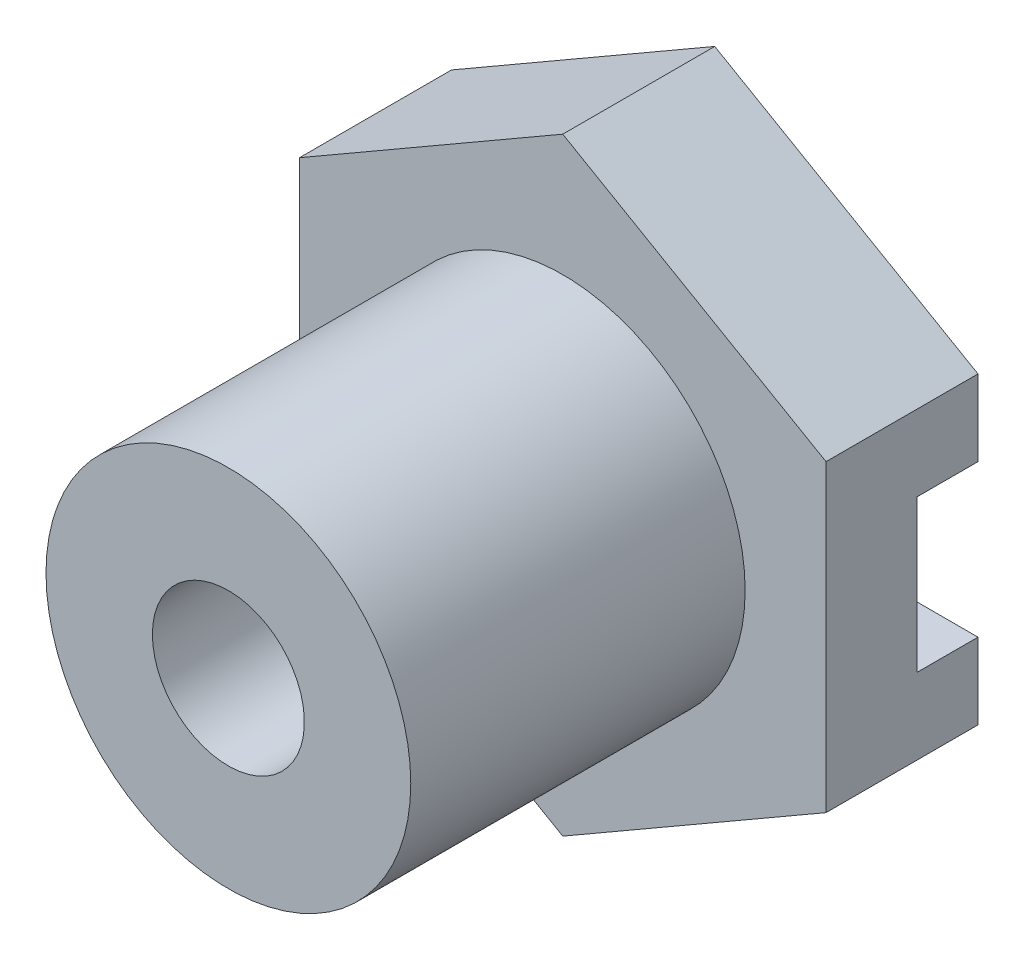
from build123d import *

# Parameters (mm, degrees)
HEX_FLANGE_DEPTH          = 5
BOSS_SKETCH_12_R          = 6
CYLINDRICAL_BOSS_12_DEPTH = 11
FLANGE_SLOT_SKETCH_W      = 17.320508076
FLANGE_SLOT_SKETCH_H      = 5
FLANGE_SLOT_CUT_DEPTH     = 2
BORE_SKETCH_5_R           = 2.5
BORE_5_DEPTH              = 20.261360284


with BuildPart() as part:
    # Hex Flange Sketch → Hex Flange (new body)
    with BuildSketch(Plane.XY):
        Polygon((0, 10), (-8.660254038, 5), (-8.660254038, -5), (0, -10), (8.660254038, -5), (8.660254038, 5), align=None)
    extrude(amount=HEX_FLANGE_DEPTH)

    # Boss Sketch Ø12 → Cylindrical Boss Ø12 (add)
    with BuildSketch(Plane.XY.offset(5)):
        Circle(BOSS_SKETCH_12_R)
    extrude(amount=CYLINDRICAL_BOSS_12_DEPTH)

    # Flange Slot Sketch → Flange Slot Cut (cut)
    with BuildSketch(Plane(origin=(0, 0, 0), x_dir=(-1, 0, 0), z_dir=(0, 0, -1))):
        Rectangle(FLANGE_SLOT_SKETCH_W, FLANGE_SLOT_SKETCH_H)
    extrude(amount=-FLANGE_SLOT_CUT_DEPTH, mode=Mode.SUBTRACT)

    # Bore Sketch Ø5 → Bore Ø5 (cut, through all)
    with BuildSketch(Plane(origin=(0, 0, 2), x_dir=(-1, 0, 0), z_dir=(0, 0, -1))):
        Circle(BORE_SKETCH_5_R)
    extrude(amount=-BORE_5_DEPTH, mode=Mode.SUBTRACT)


solid = part.part
